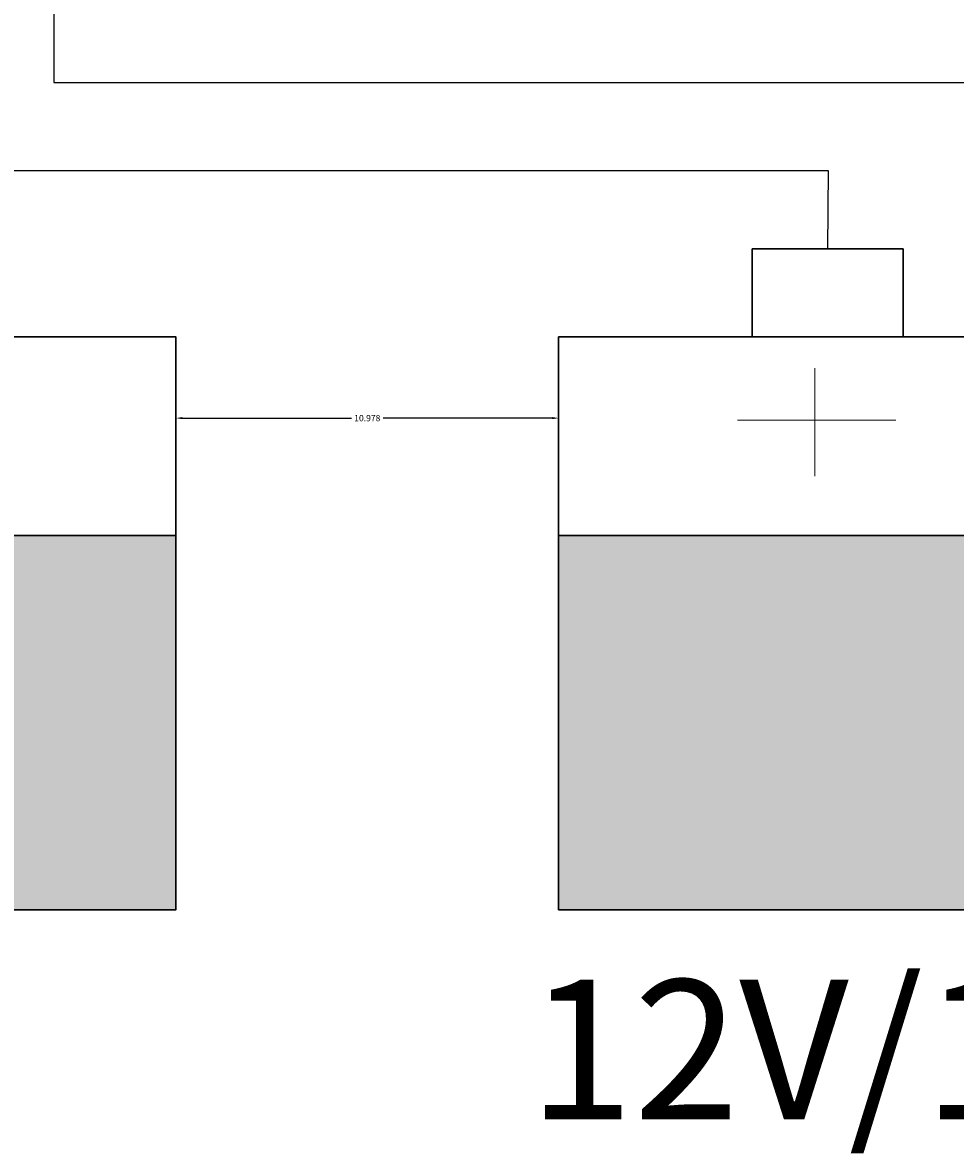
# Model space of a CAD drawing. Units: millimetres. Extents: x -8 to 285, y 5 to 221.
# Tile 3 of 30: x 57 to 84, y 13 to 45. Entities that reach past the tile are written whole.
import ezdxf

# ---------------------------------------------------------------- set-up
doc = ezdxf.new("R2010")
doc.units = ezdxf.units.MM
for name, color, linetype, lineweight in [('A-ANNO-DIMS', 2, 'Continuous', 18), ('E-ANNO-SYMB', 7, 'Continuous', 18), ('E-ANNO-TEXT', 7, 'Continuous', 18), ('E-EQPM-PATT', 252, 'Continuous', 13), ('E-POWR-BATT', 7, 'Continuous', 30), ('E-POWR-DC-LINK', 4, 'Continuous', 25), ('E-POWR-DC-NEG', 3, 'Continuous', 25)]:
    doc.layers.add(name, color=color, linetype=linetype, lineweight=lineweight)
doc.styles.get("Standard").update_dxf_attribs({"font": 'arial.ttf'})
doc.dimstyles.get("Standard").update_dxf_attribs({"dimtxt": 0.18, "dimasz": 0.18, "dimexe": 0.18, "dimexo": 0.0625, "dimgap": 0.09, "dimtad": 0, "dimtih": 1, "dimtoh": 1, "dimdec": 4, "dimzin": 0, "dimdsep": 46, "dimtxsty": 'Standard', "dimcen": 0.09, "dimadec": 0, "dimazin": 0, "dimtfac": 1, "dimtdec": 4, "dimtofl": 0, "dimtmove": 0, "dimatfit": 3, "dimfxl": 1, "dimtolj": 1, "dimtzin": 0, "dimarcsym": 0})

# ---------------------------------------------------------------- blocks, each defined once
blk = doc.blocks.new('BATTERY-CASE')
blk.add_line((0, 10.738), (31.163, 10.738))
blk.add_lwpolyline([(0, 16.427), (31.163, 16.427), (31.163, 0), (0, 0)], close=True)
blk = doc.blocks.new('BATTERY-TERMINAL-POST')
for p, q in [((0, 0), (0, 2.525)), ((0, 2.525), (4.334, 2.525)), ((4.334, 2.525), (4.334, 0))]:
    blk.add_line(p, q)
blk = doc.blocks.new('POLARITY-POSITIVE')
for p, q in [((2.22, 3.095), (2.22, 0)), ((0, 1.599), (4.543, 1.599))]:
    blk.add_line(p, q)
blk = doc.blocks.new('*D10')
at = {"layer": 'A-ANNO-DIMS', "color": 0, "lineweight": -2, "transparency": 16777216}
for p, q in [((145.103, 206.457), (-7.608, 206.457)), ((-7.428, 206.277), (-7.428, 113.161)), ((-7.428, 19.682), (-7.428, 112.797)), ((30.453, 19.502), (-7.608, 19.502))]:
    blk.add_line(p, q, dxfattribs=at)
at = {"layer": 'A-ANNO-DIMS', "color": 0, "transparency": 16777216}
for points in [[(-7.458, 206.277), (-7.398, 206.277), (-7.428, 206.457)], [(-7.458, 19.682), (-7.398, 19.682), (-7.428, 19.502)]]:
    blk.add_solid(points, dxfattribs=at)
at = {"layer": 'Defpoints', "color": 0, "transparency": 16777216}
for p in [(-7.428, 206.457), (145.165, 206.457), (30.516, 19.502)]:
    blk.add_point(p, dxfattribs=at)
at = {"layer": 'A-ANNO-DIMS', "color": 0, "transparency": 16777216, "insert": (-7.428, 112.979), "char_height": 0.18, "attachment_point": 5}
blk.add_mtext('\\A1;186.95', dxfattribs=at)
blk = doc.blocks.new('*D23')
at = {"layer": 'A-ANNO-DIMS', "color": 0, "lineweight": -2, "transparency": 16777216}
for p, q in [((61.679, 19.564), (61.679, 33.782)), ((72.657, 19.564), (72.657, 33.782)), ((61.859, 33.602), (66.712, 33.602)), ((72.477, 33.602), (67.623, 33.602))]:
    blk.add_line(p, q, dxfattribs=at)
at = {"layer": 'A-ANNO-DIMS', "color": 0, "transparency": 16777216}
for points in [[(61.859, 33.632), (61.859, 33.572), (61.679, 33.602)], [(72.477, 33.632), (72.477, 33.572), (72.657, 33.602)]]:
    blk.add_solid(points, dxfattribs=at)
at = {"layer": 'Defpoints', "color": 0, "transparency": 16777216}
for p in [(72.657, 33.602), (61.679, 19.502), (72.657, 19.502)]:
    blk.add_point(p, dxfattribs=at)
at = {"layer": 'A-ANNO-DIMS', "color": 0, "transparency": 16777216, "insert": (67.168, 33.602), "char_height": 0.18, "attachment_point": 5}
blk.add_mtext('\\A1;10.978', dxfattribs=at)

msp = doc.modelspace()

# ---------------------------------------------------------------- hatches: boundary and pattern name
at = {"layer": 'E-EQPM-PATT'}
h = msp.add_hatch(color=256, dxfattribs=at)
h.set_gradient(color1=(244, 238, 81), color2=(248, 153, 30), tint=1)
h.paths.add_polyline_path([(30.516, 30.2396), (30.516, 19.502), (61.6786, 19.502), (61.6786, 30.2396)])
h.paths.add_polyline_path([(44.6613, 24.9143), (46.8335, 24.9143), (44.845, 28.3584), (45.9646, 28.3584), (50.1024, 23.1306), (46.8299, 24.1393), (47.652, 20.7882)], flags=16)
h.paths.add_polyline_path([(72.6568, 30.2396), (72.6568, 19.502), (103.8194, 19.502), (103.8194, 30.2396)])
h.paths.add_polyline_path([(86.2008, 24.9143), (88.373, 24.9143), (86.3846, 28.3584), (87.5041, 28.3584), (91.6419, 23.1306), (88.3694, 24.1393), (89.1915, 20.7882)], flags=16)

# ---------------------------------------------------------------- linework, layer by layer
at = {"layer": 'E-POWR-DC-LINK'}
msp.add_lwpolyline([(50.7659, 40.7074), (80.3875, 40.7074), (80.3759, 38.4537)], dxfattribs=at)
at = {"layer": 'E-POWR-DC-NEG'}
msp.add_lwpolyline([(58.1717, 67.9064), (58.1717, 43.2239), (94.0348, 43.2239), (94.1079, 38.4537)], dxfattribs=at)

# ---------------------------------------------------------------- block references
at = {"layer": 'E-ANNO-SYMB'}
msp.add_blockref('POLARITY-POSITIVE', (77.7876, 31.94), dxfattribs=at)
at = {"layer": 'E-POWR-BATT'}
for name, p in [('BATTERY-TERMINAL-POST', (78.2091, 35.929)), ('BATTERY-CASE', (30.516, 19.502)), ('BATTERY-CASE', (72.6568, 19.502))]:
    msp.add_blockref(name, p, dxfattribs=at)

# ---------------------------------------------------------------- texts
at = {"layer": 'E-ANNO-TEXT', "insert": (33.3813, 17.4943), "char_height": 4, "attachment_point": 1}
msp.add_mtext_dynamic_manual_height_columns('12V/100h            12V/100Ah', width=74.08228, gutter_width=12.5, heights=[0], dxfattribs=at)

# ---------------------------------------------------------------- dimensions: what is measured, and where the dimension line sits
at = {"layer": 'A-ANNO-DIMS'}
dim = msp.add_linear_dim(base=(-7.4275, 206.4568), p1=(30.516, 19.502), p2=(145.1651, 206.4568), angle=90, dimstyle='Standard', override={"dimdec": 2, "dimlfac": 1, "dimrnd": 0, "dimzin": 0, "dimdsep": 46, "dimlunit": 2}, dxfattribs=at)
dim.commit()
dim.dimension.update_dxf_attribs({"geometry": '*D10', "text_midpoint": (-7.4275, 112.9794)})
dim = msp.add_linear_dim(base=(72.6568, 33.602), p1=(61.6786, 19.502), p2=(72.6568, 19.502), dimstyle='Standard', override={"dimdec": 3, "dimlfac": 1, "dimrnd": 0, "dimzin": 0, "dimdsep": 46, "dimlunit": 2}, dxfattribs=at)
dim.commit()
dim.dimension.update_dxf_attribs({"geometry": '*D23', "text_midpoint": (67.1677, 33.602)})

doc.saveas('drawing.dxf')
